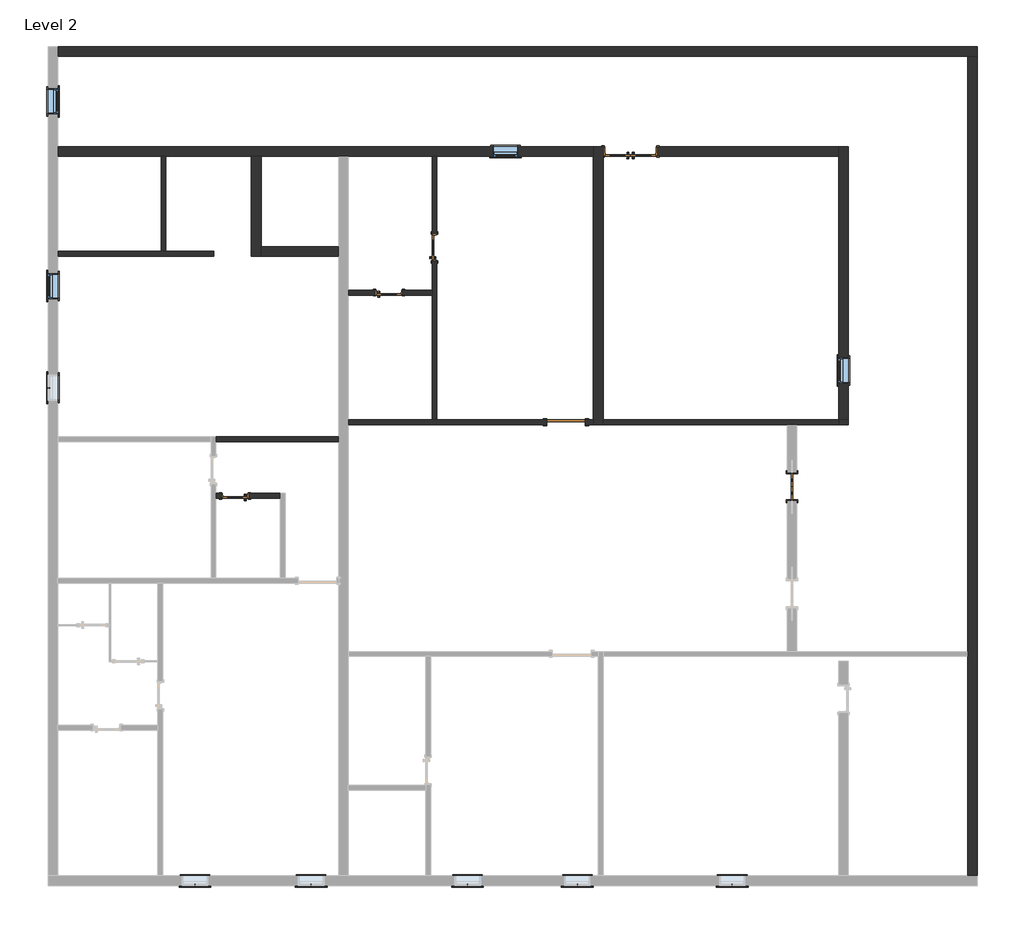
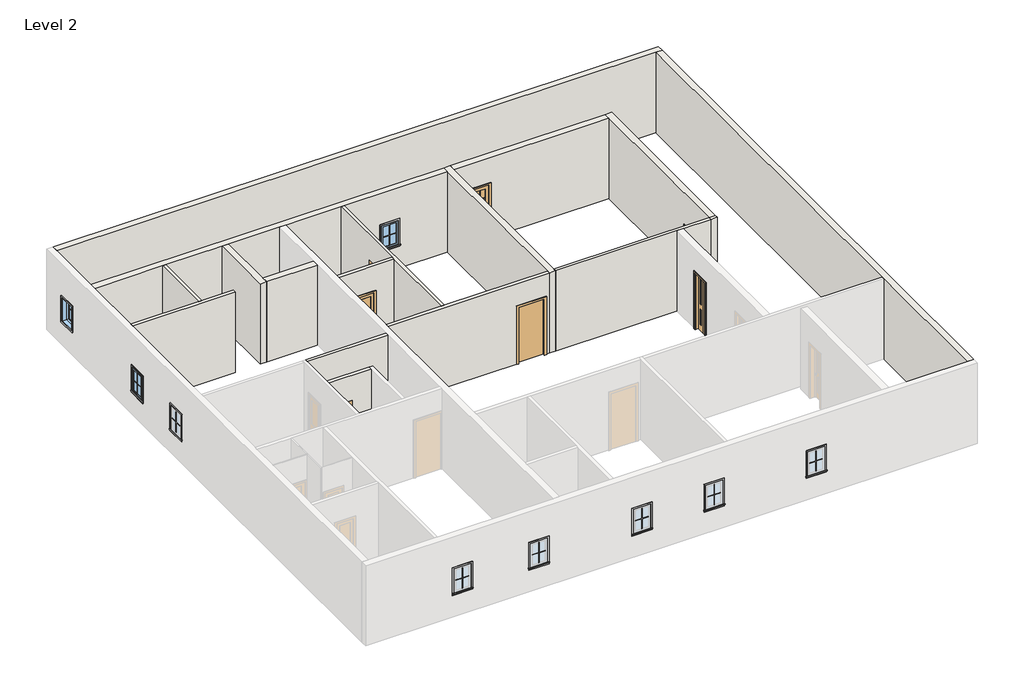
# One storey, part 2 of 2: 30 proxies, 17 walls, 6 doors, 4 windows.
"""IFC4 building model written with IfcOpenShell, lengths in millimetres."""

from ifc_helpers import new_model, si_unit, frame, origin, place, context, project, spatial, polyline, outline, extrude, faceted_brep, transform, mapped, element, save
from components import muntin_pattern_2x2_muntin_pattern_2x2_cf4092f1, muntin_pattern_2x2_muntin_pattern_2x2_49143b38, trim_window_exterior_flat_with_sill_a665a915, trim_window_exterior_flat_with_sill_4c72db77, trim_window_interior_flat_picture_frame_d485c387, trim_window_interior_flat_picture_frame_dfd23ff3, door_cd3c5da8, door_interior_double_pocket_2_panel_wood_door_interior_52fbc1e8, door_interior_single_2_panel_wood_door_interior_single_2_a051e6ed, door_interior_single_2_panel_wood_door_interior_single_2_03d66c98, door_e5f9f3c4, window_bab9308a

model = new_model("IFC4")

# Units and contexts
model_context = context("Model", 3, world=origin())
ifc_project = project(units=[si_unit("LENGTHUNIT", "METRE", prefix="MILLI")], contexts=[model_context])

# Site, building, storey
site = spatial("IfcSite", under=ifc_project)
building = spatial("IfcBuilding", under=site)
storey = spatial("IfcBuildingStorey", under=building, Name="Level 2", Elevation=457.2)

# Proxies
placement = place(None, origin())
muntin_pattern_2x2_muntin_pattern_2x2_shape = muntin_pattern_2x2_muntin_pattern_2x2_cf4092f1(model_context)
element("IfcBuildingElementProxy", 1, Name="Muntin Pattern_2x2 : Muntin Pattern_2x2", ObjectType="Muntin Pattern_2x2 : Muntin Pattern_2x2", at=placement, inside=storey, context=model_context, shape_type="MappedRepresentation", body=[
    mapped(muntin_pattern_2x2_muntin_pattern_2x2_shape, transform((536.9549703, -9076.4534081, 1441.45), x_axis=(-1.0, 0.0, 0.0), y_axis=(0.0, -1.0, 0.0), z_axis=(0.0, 0.0, 1.0))),
])
element("IfcBuildingElementProxy", 2, Name="Muntin Pattern_2x2 : Muntin Pattern_2x2", ObjectType="Muntin Pattern_2x2 : Muntin Pattern_2x2", at=placement, inside=storey, context=model_context, shape_type="MappedRepresentation", body=[
    mapped(muntin_pattern_2x2_muntin_pattern_2x2_shape, transform((-2053.8450297, -9076.4534081, 1441.45), x_axis=(-1.0, 0.0, 0.0), y_axis=(0.0, -1.0, 0.0), z_axis=(0.0, 0.0, 1.0))),
])
element("IfcBuildingElementProxy", 3, Name="Muntin Pattern_2x2 : Muntin Pattern_2x2", ObjectType="Muntin Pattern_2x2 : Muntin Pattern_2x2", at=placement, inside=storey, context=model_context, shape_type="MappedRepresentation", body=[
    mapped(muntin_pattern_2x2_muntin_pattern_2x2_shape, transform((-5749.5450297, -9076.4534081, 1441.45), x_axis=(-1.0, 0.0, 0.0), y_axis=(0.0, -1.0, 0.0), z_axis=(0.0, 0.0, 1.0))),
])
element("IfcBuildingElementProxy", 4, Name="Muntin Pattern_2x2 : Muntin Pattern_2x2", ObjectType="Muntin Pattern_2x2 : Muntin Pattern_2x2", at=placement, inside=storey, context=model_context, shape_type="MappedRepresentation", body=[
    mapped(muntin_pattern_2x2_muntin_pattern_2x2_shape, transform((-8492.7450297, -9076.4534081, 1441.45), x_axis=(-1.0, 0.0, 0.0), y_axis=(0.0, -1.0, 0.0), z_axis=(0.0, 0.0, 1.0))),
])
element("IfcBuildingElementProxy", 5, Name="Muntin Pattern_2x2 : Muntin Pattern_2x2", ObjectType="Muntin Pattern_2x2 : Muntin Pattern_2x2", at=placement, inside=storey, context=model_context, shape_type="MappedRepresentation", body=[
    mapped(muntin_pattern_2x2_muntin_pattern_2x2_shape, transform((-11740.7700297, 9432.2090919, 1441.45), x_axis=(0.0, -1.0, 0.0), y_axis=(1.0, 0.0, 0.0), z_axis=(0.0, 0.0, 1.0))),
])
element("IfcBuildingElementProxy", 6, Name="Muntin Pattern_2x2 : Muntin Pattern_2x2", ObjectType="Muntin Pattern_2x2 : Muntin Pattern_2x2", at=placement, inside=storey, context=model_context, shape_type="MappedRepresentation", body=[
    mapped(muntin_pattern_2x2_muntin_pattern_2x2_shape, transform((-11950.3200297, 5069.7590919, 1441.45), x_axis=(0.0, 1.0, 0.0), y_axis=(-1.0, 0.0, 0.0), z_axis=(0.0, 0.0, 1.0))),
])
element("IfcBuildingElementProxy", 7, Name="Muntin Pattern_2x2 : Muntin Pattern_2x2", ObjectType="Muntin Pattern_2x2 : Muntin Pattern_2x2", at=placement, inside=storey, context=model_context, shape_type="MappedRepresentation", body=[
    mapped(muntin_pattern_2x2_muntin_pattern_2x2_shape, transform((-11950.3200297, 2669.4590919, 1441.45), x_axis=(0.0, 1.0, 0.0), y_axis=(-1.0, 0.0, 0.0), z_axis=(0.0, 0.0, 1.0))),
])
element("IfcBuildingElementProxy", 8, Name="Muntin Pattern_2x2 : Muntin Pattern_2x2", ObjectType="Muntin Pattern_2x2 : Muntin Pattern_2x2", at=placement, inside=storey, context=model_context, shape_type="MappedRepresentation", body=[
    mapped(muntin_pattern_2x2_muntin_pattern_2x2_shape, transform((-1158.4950297, 8146.3340919, 1441.45), x_axis=(-1.0, 0.0, 0.0), y_axis=(0.0, -1.0, 0.0), z_axis=(0.0, 0.0, 1.0))),
])
element("IfcBuildingElementProxy", 9, Name="Muntin Pattern_2x2 : Muntin Pattern_2x2", ObjectType="Muntin Pattern_2x2 : Muntin Pattern_2x2", at=placement, inside=storey, context=model_context, shape_type="MappedRepresentation", body=[
    mapped(muntin_pattern_2x2_muntin_pattern_2x2_shape, transform((6718.6799703, 3075.8590919, 1441.45), x_axis=(0.0, 1.0, 0.0), y_axis=(-1.0, 0.0, 0.0), z_axis=(0.0, 0.0, 1.0))),
])
muntin_pattern_2x2_muntin_pattern_2x2_2_shape = muntin_pattern_2x2_muntin_pattern_2x2_49143b38(model_context)
element("IfcBuildingElementProxy", 10, Name="Muntin Pattern_2x2 : Muntin Pattern_2x2", ObjectType="Muntin Pattern_2x2 : Muntin Pattern_2x2", at=placement, inside=storey, context=model_context, shape_type="MappedRepresentation", body=[
    mapped(muntin_pattern_2x2_muntin_pattern_2x2_2_shape, transform((4194.5549703, -9076.4534081, 1441.45), x_axis=(1.0, 0.0, 0.0), y_axis=(0.0, 1.0, 0.0), z_axis=(0.0, 0.0, 1.0))),
])
trim_window_exterior_flat_with_sill_shape = trim_window_exterior_flat_with_sill_a665a915(model_context)
element("IfcBuildingElementProxy", 11, Name="Trim-Window-Exterior-Flat : with Sill", ObjectType="Trim-Window-Exterior-Flat : with Sill", at=placement, inside=storey, context=model_context, shape_type="MappedRepresentation", body=[
    mapped(trim_window_exterior_flat_with_sill_shape, transform((536.9549703, -9085.9784081, 2286.0), x_axis=(1.0, 0.0, 0.0), y_axis=(0.0, 0.0, 1.0), z_axis=(0.0, -1.0, 0.0))),
])
element("IfcBuildingElementProxy", 12, Name="Trim-Window-Exterior-Flat : with Sill", ObjectType="Trim-Window-Exterior-Flat : with Sill", at=placement, inside=storey, context=model_context, shape_type="MappedRepresentation", body=[
    mapped(trim_window_exterior_flat_with_sill_shape, transform((-2053.8450297, -9085.9784081, 2286.0), x_axis=(1.0, 0.0, 0.0), y_axis=(0.0, 0.0, 1.0), z_axis=(0.0, -1.0, 0.0))),
])
element("IfcBuildingElementProxy", 13, Name="Trim-Window-Exterior-Flat : with Sill", ObjectType="Trim-Window-Exterior-Flat : with Sill", at=placement, inside=storey, context=model_context, shape_type="MappedRepresentation", body=[
    mapped(trim_window_exterior_flat_with_sill_shape, transform((-5749.5450297, -9085.9784081, 2286.0), x_axis=(1.0, 0.0, 0.0), y_axis=(0.0, 0.0, 1.0), z_axis=(0.0, -1.0, 0.0))),
])
element("IfcBuildingElementProxy", 14, Name="Trim-Window-Exterior-Flat : with Sill", ObjectType="Trim-Window-Exterior-Flat : with Sill", at=placement, inside=storey, context=model_context, shape_type="MappedRepresentation", body=[
    mapped(trim_window_exterior_flat_with_sill_shape, transform((-8492.7450297, -9085.9784081, 2286.0), x_axis=(1.0, 0.0, 0.0), y_axis=(0.0, 0.0, 1.0), z_axis=(0.0, -1.0, 0.0))),
])
element("IfcBuildingElementProxy", 15, Name="Trim-Window-Exterior-Flat : with Sill", ObjectType="Trim-Window-Exterior-Flat : with Sill", at=placement, inside=storey, context=model_context, shape_type="MappedRepresentation", body=[
    mapped(trim_window_exterior_flat_with_sill_shape, transform((-11731.2450297, 9432.2090919, 2286.0), x_axis=(0.0, 1.0, 0.0), y_axis=(0.0, 0.0, 1.0), z_axis=(1.0, 0.0, 0.0))),
])
element("IfcBuildingElementProxy", 16, Name="Trim-Window-Exterior-Flat : with Sill", ObjectType="Trim-Window-Exterior-Flat : with Sill", at=placement, inside=storey, context=model_context, shape_type="MappedRepresentation", body=[
    mapped(trim_window_exterior_flat_with_sill_shape, transform((-11959.8450297, 5069.7590919, 2286.0), x_axis=(0.0, -1.0, 0.0), y_axis=(0.0, 0.0, 1.0), z_axis=(-1.0, 0.0, 0.0))),
])
element("IfcBuildingElementProxy", 17, Name="Trim-Window-Exterior-Flat : with Sill", ObjectType="Trim-Window-Exterior-Flat : with Sill", at=placement, inside=storey, context=model_context, shape_type="MappedRepresentation", body=[
    mapped(trim_window_exterior_flat_with_sill_shape, transform((-11959.8450297, 2669.4590919, 2286.0), x_axis=(0.0, -1.0, 0.0), y_axis=(0.0, 0.0, 1.0), z_axis=(-1.0, 0.0, 0.0))),
])
element("IfcBuildingElementProxy", 18, Name="Trim-Window-Exterior-Flat : with Sill", ObjectType="Trim-Window-Exterior-Flat : with Sill", at=placement, inside=storey, context=model_context, shape_type="MappedRepresentation", body=[
    mapped(trim_window_exterior_flat_with_sill_shape, transform((-1158.4950297, 8136.8090919, 2286.0), x_axis=(1.0, 0.0, 0.0), y_axis=(0.0, 0.0, 1.0), z_axis=(0.0, -1.0, 0.0))),
])
element("IfcBuildingElementProxy", 19, Name="Trim-Window-Exterior-Flat : with Sill", ObjectType="Trim-Window-Exterior-Flat : with Sill", at=placement, inside=storey, context=model_context, shape_type="MappedRepresentation", body=[
    mapped(trim_window_exterior_flat_with_sill_shape, transform((6709.1549703, 3075.8590919, 2286.0), x_axis=(0.0, -1.0, 0.0), y_axis=(0.0, 0.0, 1.0), z_axis=(-1.0, 0.0, 0.0))),
])
trim_window_exterior_flat_with_sill_2_shape = trim_window_exterior_flat_with_sill_4c72db77(model_context)
element("IfcBuildingElementProxy", 20, Name="Trim-Window-Exterior-Flat : with Sill", ObjectType="Trim-Window-Exterior-Flat : with Sill", at=placement, inside=storey, context=model_context, shape_type="MappedRepresentation", body=[
    mapped(trim_window_exterior_flat_with_sill_2_shape, transform((4194.5549703, -9085.9784081, 2286.0), x_axis=(-1.0, 0.0, 0.0), y_axis=(0.0, 0.0, -1.0), z_axis=(0.0, -1.0, 0.0))),
])
trim_window_interior_flat_picture_frame_shape = trim_window_interior_flat_picture_frame_d485c387(model_context)
element("IfcBuildingElementProxy", 21, Name="Trim-Window-Interior-Flat : Picture Frame", ObjectType="Trim-Window-Interior-Flat : Picture Frame", at=placement, inside=storey, context=model_context, shape_type="MappedRepresentation", body=[
    mapped(trim_window_interior_flat_picture_frame_shape, transform((536.9549703, -8857.3784081, 2286.0), x_axis=(-1.0, 0.0, 0.0), y_axis=(0.0, 0.0, 1.0), z_axis=(0.0, 1.0, 0.0))),
])
element("IfcBuildingElementProxy", 22, Name="Trim-Window-Interior-Flat : Picture Frame", ObjectType="Trim-Window-Interior-Flat : Picture Frame", at=placement, inside=storey, context=model_context, shape_type="MappedRepresentation", body=[
    mapped(trim_window_interior_flat_picture_frame_shape, transform((-2053.8450297, -8857.3784081, 2286.0), x_axis=(-1.0, 0.0, 0.0), y_axis=(0.0, 0.0, 1.0), z_axis=(0.0, 1.0, 0.0))),
])
element("IfcBuildingElementProxy", 23, Name="Trim-Window-Interior-Flat : Picture Frame", ObjectType="Trim-Window-Interior-Flat : Picture Frame", at=placement, inside=storey, context=model_context, shape_type="MappedRepresentation", body=[
    mapped(trim_window_interior_flat_picture_frame_shape, transform((-5749.5450297, -8857.3784081, 2286.0), x_axis=(-1.0, 0.0, 0.0), y_axis=(0.0, 0.0, 1.0), z_axis=(0.0, 1.0, 0.0))),
])
element("IfcBuildingElementProxy", 24, Name="Trim-Window-Interior-Flat : Picture Frame", ObjectType="Trim-Window-Interior-Flat : Picture Frame", at=placement, inside=storey, context=model_context, shape_type="MappedRepresentation", body=[
    mapped(trim_window_interior_flat_picture_frame_shape, transform((-8492.7450297, -8857.3784081, 2286.0), x_axis=(-1.0, 0.0, 0.0), y_axis=(0.0, 0.0, 1.0), z_axis=(0.0, 1.0, 0.0))),
])
element("IfcBuildingElementProxy", 25, Name="Trim-Window-Interior-Flat : Picture Frame", ObjectType="Trim-Window-Interior-Flat : Picture Frame", at=placement, inside=storey, context=model_context, shape_type="MappedRepresentation", body=[
    mapped(trim_window_interior_flat_picture_frame_shape, transform((-11959.8450297, 9432.2090919, 2286.0), x_axis=(0.0, -1.0, 0.0), y_axis=(0.0, 0.0, 1.0), z_axis=(-1.0, 0.0, 0.0))),
])
element("IfcBuildingElementProxy", 26, Name="Trim-Window-Interior-Flat : Picture Frame", ObjectType="Trim-Window-Interior-Flat : Picture Frame", at=placement, inside=storey, context=model_context, shape_type="MappedRepresentation", body=[
    mapped(trim_window_interior_flat_picture_frame_shape, transform((-11731.2450297, 5069.7590919, 2286.0), x_axis=(0.0, 1.0, 0.0), y_axis=(0.0, 0.0, 1.0), z_axis=(1.0, 0.0, 0.0))),
])
element("IfcBuildingElementProxy", 27, Name="Trim-Window-Interior-Flat : Picture Frame", ObjectType="Trim-Window-Interior-Flat : Picture Frame", at=placement, inside=storey, context=model_context, shape_type="MappedRepresentation", body=[
    mapped(trim_window_interior_flat_picture_frame_shape, transform((-11731.2450297, 2669.4590919, 2286.0), x_axis=(0.0, 1.0, 0.0), y_axis=(0.0, 0.0, 1.0), z_axis=(1.0, 0.0, 0.0))),
])
element("IfcBuildingElementProxy", 28, Name="Trim-Window-Interior-Flat : Picture Frame", ObjectType="Trim-Window-Interior-Flat : Picture Frame", at=placement, inside=storey, context=model_context, shape_type="MappedRepresentation", body=[
    mapped(trim_window_interior_flat_picture_frame_shape, transform((-1158.4950297, 8365.4090919, 2286.0), x_axis=(-1.0, 0.0, 0.0), y_axis=(0.0, 0.0, 1.0), z_axis=(0.0, 1.0, 0.0))),
])
element("IfcBuildingElementProxy", 29, Name="Trim-Window-Interior-Flat : Picture Frame", ObjectType="Trim-Window-Interior-Flat : Picture Frame", at=placement, inside=storey, context=model_context, shape_type="MappedRepresentation", body=[
    mapped(trim_window_interior_flat_picture_frame_shape, transform((6937.7549703, 3075.8590919, 2286.0), x_axis=(0.0, 1.0, 0.0), y_axis=(0.0, 0.0, 1.0), z_axis=(1.0, 0.0, 0.0))),
])
trim_window_interior_flat_picture_frame_2_shape = trim_window_interior_flat_picture_frame_dfd23ff3(model_context)
element("IfcBuildingElementProxy", 30, Name="Trim-Window-Interior-Flat : Picture Frame", ObjectType="Trim-Window-Interior-Flat : Picture Frame", at=placement, inside=storey, context=model_context, shape_type="MappedRepresentation", body=[
    mapped(trim_window_interior_flat_picture_frame_2_shape, transform((4194.5549703, -8857.3784081, 2286.0), x_axis=(1.0, 0.0, 0.0), y_axis=(0.0, 0.0, -1.0), z_axis=(0.0, 1.0, 0.0))),
])

# Doors
door_shape = door_cd3c5da8(model_context)
element("IfcDoor", 31, ObjectType="Door-Interior-Double-Full Glass-Wood : 48\" x 80\"", at=placement, inside=storey, context=model_context, shape_type="MappedRepresentation", body=[
    mapped(door_shape, transform((1794.2549703, 8247.9340919, 457.2), x_axis=(-1.0, 0.0, 0.0), y_axis=(0.0, -1.0, 0.0), z_axis=(0.0, 0.0, 1.0))),
])
door_interior_double_pocket_2_panel_wood_door_interior_shape = door_interior_double_pocket_2_panel_wood_door_interior_52fbc1e8(model_context)
element("IfcDoor", 32, ObjectType="Door-Interior-Double-Pocket-2_Panel-Wood : Door-Interior-Double-Pocket-2_Panel-Wood", at=placement, inside=storey, context=model_context, shape_type="MappedRepresentation", body=[
    mapped(door_interior_double_pocket_2_panel_wood_door_interior_shape, transform((5604.2549703, 332.6590919, 457.2), x_axis=(0.0, -1.0, 0.0), y_axis=(1.0, 0.0, 0.0), z_axis=(0.0, 0.0, 1.0))),
])
door_interior_single_2_panel_wood_door_interior_single_2_shape = door_interior_single_2_panel_wood_door_interior_single_2_a051e6ed(model_context)
element("IfcDoor", 33, ObjectType="Door-Interior-Single-2_Panel-Wood : Door-Interior-Single-2_Panel-Wood", at=placement, inside=storey, context=model_context, shape_type="MappedRepresentation", body=[
    mapped(door_interior_single_2_panel_wood_door_interior_single_2_shape, transform((-7546.5950297, 113.5840919, 457.2), x_axis=(-1.0, 0.0, 0.0), y_axis=(0.0, -1.0, 0.0), z_axis=(0.0, 0.0, 1.0))),
])
element("IfcDoor", 34, ObjectType="Door-Interior-Single-2_Panel-Wood : d3", at=placement, inside=storey, context=model_context, shape_type="MappedRepresentation", body=[
    mapped(door_interior_single_2_panel_wood_door_interior_single_2_shape, transform((-2838.0700297, 5984.1590919, 457.2), x_axis=(0.0, 1.0, 0.0), y_axis=(-1.0, 0.0, 0.0), z_axis=(0.0, 0.0, 1.0))),
])
door_interior_single_2_panel_wood_door_interior_single_2_2_shape = door_interior_single_2_panel_wood_door_interior_single_2_03d66c98(model_context)
element("IfcDoor", 35, ObjectType="Door-Interior-Single-2_Panel-Wood : d3", at=placement, inside=storey, context=model_context, shape_type="MappedRepresentation", body=[
    mapped(door_interior_single_2_panel_wood_door_interior_single_2_2_shape, transform((-3911.2200297, 4914.1840919, 457.2), x_axis=(1.0, 0.0, 0.0), y_axis=(0.0, 1.0, 0.0), z_axis=(0.0, 0.0, 1.0))),
])
door_2_shape = door_e5f9f3c4(model_context)
element("IfcDoor", 36, ObjectType="Single-Flush : 36\" x 84\"", at=placement, inside=storey, context=model_context, shape_type="MappedRepresentation", body=[
    mapped(door_2_shape, transform((270.2549703, 1856.6590919, 457.2), x_axis=(1.0, 0.0, 0.0), y_axis=(0.0, 1.0, 0.0), z_axis=(0.0, 0.0, 1.0))),
])

# Walls
element("IfcWall", 37, ObjectType="4.5\" wall", at=placement, inside=storey, context=model_context, shape_type="SweptSolid", body=[
    extrude(outline(polyline([(3505.2, -6473.4450297), (3505.2, -7997.4450297), (457.2, -7997.4450297), (457.2, -7876.7950297), (2514.6, -7876.7950297), (2514.6, -7216.3950297), (457.2, -7216.3950297), (457.2, -6473.4450297), (3505.2, -6473.4450297)])), frame((0.0, 59.6090919, 0.0), z_axis=(0.0, 1.0, 0.0), x_axis=(0.0, 0.0, 1.0)), (0.0, 0.0, 1.0), 114.3),
])
element("IfcWall", 38, ObjectType="4.5\" wall", at=placement, inside=storey, context=model_context, shape_type="SweptSolid", body=[
    extrude(outline(polyline([(-7997.4450297, 1507.4090919), (-5101.8450297, 1507.4090919), (-5101.8450297, 1393.1090919), (-7997.4450297, 1393.1090919), (-7997.4450297, 1507.4090919)])), frame((0.0, 0.0, 457.2), z_axis=(0.0, 0.0, 1.0), x_axis=(1.0, 0.0, 0.0)), (0.0, 0.0, 1.0), 3048.0),
])
element("IfcWall", 39, ObjectType="4.5\" wall", at=placement, inside=storey, context=model_context, shape_type="Brep", body=[
    faceted_brep([(-2892.0450297, 1913.8090919, 3505.2), (-2892.0450297, 4860.2090919, 3505.2), (-2892.0450297, 4974.5090919, 3505.2), (-2892.0450297, 8136.8090919, 3505.2), (-2892.0450297, 8136.8090919, 457.2), (-2892.0450297, 6314.3590919, 457.2), (-2892.0450297, 6314.3590919, 2514.6), (-2892.0450297, 5653.9590919, 2514.6), (-2892.0450297, 5653.9590919, 457.2), (-2892.0450297, 4974.5090919, 457.2), (-2892.0450297, 4860.2090919, 457.2), (-2892.0450297, 1913.8090919, 457.2), (-2777.7450297, 8136.8090919, 3505.2), (-2777.7450297, 1913.8090919, 3505.2), (-2777.7450297, 1913.8090919, 457.2), (-2777.7450297, 5653.9590919, 457.2), (-2777.7450297, 5653.9590919, 2514.6), (-2777.7450297, 6314.3590919, 2514.6), (-2777.7450297, 6314.3590919, 457.2), (-2777.7450297, 8136.8090919, 457.2)], [[[0, 1, 2, 3, 4, 5, 6, 7, 8, 9, 10, 11]], [[12, 13, 14, 15, 16, 17, 18, 19]], [[4, 19, 18, 5]], [[14, 11, 10, 9, 8, 15]], [[3, 2, 1, 0, 13, 12]], [[4, 3, 12, 19]], [[0, 11, 14, 13]], [[17, 6, 5, 18]], [[6, 17, 16, 7]], [[7, 16, 15, 8]]]),
])
element("IfcWall", 40, ObjectType="4.5\" wall", at=placement, inside=storey, context=model_context, shape_type="Brep", body=[
    faceted_brep([(727.4549703, 1799.5090919, 2590.8), (727.4549703, 1799.5090919, 457.2), (917.9549703, 1799.5090919, 457.2), (917.9549703, 1799.5090919, 3505.2), (-4873.2450297, 1799.5090919, 3505.2), (-4873.2450297, 1799.5090919, 457.2), (-186.9450297, 1799.5090919, 457.2), (-186.9450297, 1799.5090919, 2590.8), (917.9549703, 1913.8090919, 457.2), (727.4549703, 1913.8090919, 457.2), (727.4549703, 1913.8090919, 2590.8), (-186.9450297, 1913.8090919, 2590.8), (-186.9450297, 1913.8090919, 457.2), (-2777.7450297, 1913.8090919, 457.2), (-2892.0450297, 1913.8090919, 457.2), (-4873.2450297, 1913.8090919, 457.2), (-4873.2450297, 1913.8090919, 3505.2), (-2892.0450297, 1913.8090919, 3505.2), (-2777.7450297, 1913.8090919, 3505.2), (917.9549703, 1913.8090919, 3505.2)], [[[0, 1, 2, 3, 4, 5, 6, 7]], [[8, 9, 10, 11, 12, 13, 14, 15, 16, 17, 18, 19]], [[6, 5, 15, 14, 13, 12]], [[2, 1, 9, 8]], [[4, 3, 19, 18, 17, 16]], [[5, 4, 16, 15]], [[3, 2, 8, 19]], [[10, 9, 1, 0]], [[11, 10, 0, 7]], [[12, 11, 7, 6]]]),
])
element("IfcWall", 41, ObjectType="4.5\" wall", at=placement, inside=storey, context=model_context, shape_type="SweptSolid", body=[
    extrude(outline(polyline([(3505.2, -2892.0450297), (3505.2, -4873.2450297), (457.2, -4873.2450297), (457.2, -4241.4200297), (2514.6, -4241.4200297), (2514.6, -3581.0200297), (457.2, -3581.0200297), (457.2, -2892.0450297), (3505.2, -2892.0450297)])), frame((0.0, 4860.2090919, 0.0), z_axis=(0.0, 1.0, 0.0), x_axis=(0.0, 0.0, 1.0)), (0.0, 0.0, 1.0), 114.3),
])
element("IfcWall", 42, ObjectType="4.5\" wall", at=placement, inside=storey, context=model_context, shape_type="SweptSolid", body=[
    extrude(outline(polyline([(6937.7549703, 1799.5090919), (6709.1549703, 1799.5090919), (6709.1549703, 1913.8090919), (6937.7549703, 1913.8090919), (6937.7549703, 1799.5090919)])), frame((0.0, 0.0, 457.2), z_axis=(0.0, 0.0, 1.0), x_axis=(1.0, 0.0, 0.0)), (0.0, 0.0, 1.0), 3048.0),
])
element("IfcWall", 43, ObjectType="4.5\" wall", at=placement, inside=storey, context=model_context, shape_type="Brep", body=[
    faceted_brep([(6709.1549703, 1913.8090919, 457.2), (1146.5549703, 1913.8090919, 457.2), (1146.5549703, 1913.8090919, 3505.2), (6709.1549703, 1913.8090919, 3505.2), (6709.1549703, 1799.5090919, 457.2), (6709.1549703, 1799.5090919, 3505.2), (5718.5549703, 1799.5090919, 3505.2), (5489.9549703, 1799.5090919, 3505.2), (1146.5549703, 1799.5090919, 3505.2), (1146.5549703, 1799.5090919, 457.2), (5489.9549703, 1799.5090919, 457.2), (5718.5549703, 1799.5090919, 457.2)], [[[0, 1, 2, 3]], [[4, 5, 6, 7, 8, 9, 10, 11]], [[1, 0, 4, 11, 10, 9]], [[3, 2, 8, 7, 6, 5]], [[0, 3, 5, 4]], [[2, 1, 9, 8]]]),
])
element("IfcWall", 44, ObjectType="4.5\" wall", at=placement, inside=storey, context=model_context, shape_type="SweptSolid", body=[
    extrude(outline(polyline([(-9178.5450297, 8136.8090919), (-9178.5450297, 5888.9090919), (-9292.8450297, 5888.9090919), (-9292.8450297, 8136.8090919), (-9178.5450297, 8136.8090919)])), frame((0.0, 0.0, 457.2), z_axis=(0.0, 0.0, 1.0), x_axis=(1.0, 0.0, 0.0)), (0.0, 0.0, 1.0), 3048.0),
])
element("IfcWall", 45, ObjectType="4.5\" wall", at=placement, inside=storey, context=model_context, shape_type="Brep", body=[
    faceted_brep([(-11731.2450297, 5774.6090919, 457.2), (-8051.366475, 5774.6090919, 457.2), (-8051.366475, 5774.6090919, 3505.2), (-11731.2450297, 5774.6090919, 3505.2), (-11731.2450297, 5888.9090919, 457.2), (-11731.2450297, 5888.9090919, 3505.2), (-9292.8450297, 5888.9090919, 3505.2), (-9178.5450297, 5888.9090919, 3505.2), (-8051.366475, 5888.9090919, 3505.2), (-8051.366475, 5888.9090919, 457.2), (-9178.5450297, 5888.9090919, 457.2), (-9292.8450297, 5888.9090919, 457.2)], [[[0, 1, 2, 3]], [[4, 5, 6, 7, 8, 9, 10, 11]], [[1, 0, 4, 11, 10, 9]], [[2, 1, 9, 8]], [[3, 2, 8, 7, 6, 5]], [[0, 3, 5, 4]]]),
])
element("IfcWall", 46, ObjectType="9\" wall", at=placement, inside=storey, context=model_context, shape_type="Brep", body=[
    faceted_brep([(1146.5549703, 1799.5090919, 457.2), (1146.5549703, 1913.8090919, 457.2), (1146.5549703, 8136.8090919, 457.2), (1146.5549703, 8365.4090919, 457.2), (1146.5549703, 8365.4090919, 3505.2), (1146.5549703, 8136.8090919, 3505.2), (1146.5549703, 1913.8090919, 3505.2), (1146.5549703, 1799.5090919, 3505.2), (917.9549703, 1799.5090919, 457.2), (917.9549703, 1799.5090919, 3505.2), (917.9549703, 1913.8090919, 3505.2), (917.9549703, 8136.8090919, 3505.2), (917.9549703, 8365.4090919, 3505.2), (917.9549703, 8365.4090919, 457.2), (917.9549703, 8136.8090919, 457.2), (917.9549703, 1913.8090919, 457.2)], [[[0, 1, 2, 3, 4, 5, 6, 7]], [[8, 9, 10, 11, 12, 13, 14, 15]], [[3, 2, 1, 0, 8, 15, 14, 13]], [[7, 6, 5, 4, 12, 11, 10, 9]], [[4, 3, 13, 12]], [[0, 7, 9, 8]]]),
])
element("IfcWall", 47, ObjectType="9\" wall", at=placement, inside=storey, context=model_context, shape_type="Brep", body=[
    faceted_brep([(-11731.2450297, 8136.8090919, 457.2), (-9292.8450297, 8136.8090919, 457.2), (-9178.5450297, 8136.8090919, 457.2), (-7159.2450297, 8136.8090919, 457.2), (-6930.6450297, 8136.8090919, 457.2), (-5101.8450297, 8136.8090919, 457.2), (-4873.2450297, 8136.8090919, 457.2), (-2892.0450297, 8136.8090919, 457.2), (-2777.7450297, 8136.8090919, 457.2), (917.9549703, 8136.8090919, 457.2), (917.9549703, 8136.8090919, 3505.2), (-2777.7450297, 8136.8090919, 3505.2), (-2892.0450297, 8136.8090919, 3505.2), (-4873.2450297, 8136.8090919, 3505.2), (-5101.8450297, 8136.8090919, 3505.2), (-6930.6450297, 8136.8090919, 3505.2), (-7159.2450297, 8136.8090919, 3505.2), (-9178.5450297, 8136.8090919, 3505.2), (-9292.8450297, 8136.8090919, 3505.2), (-11731.2450297, 8136.8090919, 3505.2), (-1463.2950297, 8136.8090919, 2286.0), (-853.6950297, 8136.8090919, 2286.0), (-853.6950297, 8136.8090919, 1371.6), (-1463.2950297, 8136.8090919, 1371.6), (-11731.2450297, 8365.4090919, 457.2), (-11731.2450297, 8365.4090919, 3505.2), (917.9549703, 8365.4090919, 3505.2), (917.9549703, 8365.4090919, 457.2), (-1463.2950297, 8365.4090919, 2286.0), (-1463.2950297, 8365.4090919, 1371.6), (-853.6950297, 8365.4090919, 1371.6), (-853.6950297, 8365.4090919, 2286.0)], [[[0, 1, 2, 3, 4, 5, 6, 7, 8, 9, 10, 11, 12, 13, 14, 15, 16, 17, 18, 19], [20, 21, 22, 23]], [[24, 25, 26, 27], [28, 29, 30, 31]], [[9, 8, 7, 6, 5, 4, 3, 2, 1, 0, 24, 27]], [[19, 18, 17, 16, 15, 14, 13, 12, 11, 10, 26, 25]], [[10, 9, 27, 26]], [[0, 19, 25, 24]], [[29, 28, 20, 23]], [[30, 29, 23, 22]], [[31, 30, 22, 21]], [[28, 31, 21, 20]]]),
])
element("IfcWall", 48, ObjectType="9\" wall", at=placement, inside=storey, context=model_context, shape_type="Brep", body=[
    faceted_brep([(6937.7549703, 1913.8090919, 457.2), (6937.7549703, 8365.4090919, 457.2), (6937.7549703, 8365.4090919, 3505.2), (6937.7549703, 1913.8090919, 3505.2), (6937.7549703, 3380.6590919, 2286.0), (6937.7549703, 3380.6590919, 1371.6), (6937.7549703, 2771.0590919, 1371.6), (6937.7549703, 2771.0590919, 2286.0), (6709.1549703, 1913.8090919, 457.2), (6709.1549703, 1913.8090919, 3505.2), (6709.1549703, 8136.8090919, 3505.2), (6709.1549703, 8365.4090919, 3505.2), (6709.1549703, 8365.4090919, 457.2), (6709.1549703, 8136.8090919, 457.2), (6709.1549703, 3380.6590919, 2286.0), (6709.1549703, 2771.0590919, 2286.0), (6709.1549703, 2771.0590919, 1371.6), (6709.1549703, 3380.6590919, 1371.6)], [[[0, 1, 2, 3], [4, 5, 6, 7]], [[8, 9, 10, 11, 12, 13], [14, 15, 16, 17]], [[1, 0, 8, 13, 12]], [[3, 2, 11, 10, 9]], [[2, 1, 12, 11]], [[0, 3, 9, 8]], [[5, 4, 14, 17]], [[6, 5, 17, 16]], [[7, 6, 16, 15]], [[4, 7, 15, 14]]]),
])
element("IfcWall", 49, ObjectType="9\" wall", at=placement, inside=storey, context=model_context, shape_type="SweptSolid", body=[
    extrude(outline(polyline([(3505.2, 6709.1549703), (3505.2, 1146.5549703), (457.2, 1146.5549703), (457.2, 1159.2549703), (2514.6, 1159.2549703), (2514.6, 2429.2549703), (457.2, 2429.2549703), (457.2, 6709.1549703), (3505.2, 6709.1549703)])), frame((0.0, 8136.8090919, 0.0), z_axis=(0.0, 1.0, 0.0), x_axis=(0.0, 0.0, 1.0)), (0.0, 0.0, 1.0), 228.6),
])
element("IfcWall", 50, ObjectType="9\" wall", at=placement, inside=storey, context=model_context, shape_type="Brep", body=[
    faceted_brep([(-6930.6450297, 5774.6090919, 457.2), (-6930.6450297, 6003.2090919, 457.2), (-6930.6450297, 8136.8090919, 457.2), (-6930.6450297, 8136.8090919, 3505.2), (-6930.6450297, 6003.2090919, 3505.2), (-6930.6450297, 5774.6090919, 3505.2), (-7159.2450297, 5774.6090919, 457.2), (-7159.2450297, 5774.6090919, 3505.2), (-7159.2450297, 8136.8090919, 3505.2), (-7159.2450297, 8136.8090919, 457.2)], [[[0, 1, 2, 3, 4, 5]], [[6, 7, 8, 9]], [[2, 1, 0, 6, 9]], [[5, 4, 3, 8, 7]], [[3, 2, 9, 8]], [[0, 5, 7, 6]]]),
])
element("IfcWall", 51, ObjectType="9\" wall", at=placement, inside=storey, context=model_context, shape_type="SweptSolid", body=[
    extrude(outline(polyline([(-5101.8450297, 5774.6090919), (-6930.6450297, 5774.6090919), (-6930.6450297, 6003.2090919), (-5101.8450297, 6003.2090919), (-5101.8450297, 5774.6090919)])), frame((0.0, 0.0, 457.2), z_axis=(0.0, 0.0, 1.0), x_axis=(1.0, 0.0, 0.0)), (0.0, 0.0, 1.0), 3048.0),
])
element("IfcWall", 52, ObjectType="9\" wall", at=placement, inside=storey, context=model_context, shape_type="Brep", body=[
    faceted_brep([(-11731.2450297, 10499.0090919, 457.2), (9757.1549703, 10499.0090919, 457.2), (9985.7549703, 10499.0090919, 457.2), (9985.7549703, 10499.0090919, 3505.2), (9757.1549703, 10499.0090919, 3505.2), (-11731.2450297, 10499.0090919, 3505.2), (-11731.2450297, 10727.6090919, 457.2), (-11731.2450297, 10727.6090919, 3505.2), (9985.7549703, 10727.6090919, 3505.2), (9985.7549703, 10727.6090919, 457.2)], [[[0, 1, 2, 3, 4, 5]], [[6, 7, 8, 9]], [[2, 1, 0, 6, 9]], [[5, 4, 3, 8, 7]], [[0, 5, 7, 6]], [[3, 2, 9, 8]]]),
])
element("IfcWall", 53, ObjectType="9\" wall", at=placement, inside=storey, context=model_context, shape_type="Brep", body=[
    faceted_brep([(9985.7549703, -8855.7909081, 457.2), (9985.7549703, 10499.0090919, 457.2), (9985.7549703, 10499.0090919, 3505.2), (9985.7549703, -8855.7909081, 3505.2), (9757.1549703, -8855.7909081, 457.2), (9757.1549703, -8855.7909081, 3505.2), (9757.1549703, -3674.1909081, 3505.2), (9757.1549703, -3559.8909081, 3505.2), (9757.1549703, 10499.0090919, 3505.2), (9757.1549703, 10499.0090919, 457.2), (9757.1549703, -3559.8909081, 457.2), (9757.1549703, -3674.1909081, 457.2)], [[[0, 1, 2, 3]], [[4, 5, 6, 7, 8, 9, 10, 11]], [[1, 0, 4, 11, 10, 9]], [[3, 2, 8, 7, 6, 5]], [[0, 3, 5, 4]], [[2, 1, 9, 8]]]),
])

# Windows
window_shape = window_bab9308a(model_context)
element("IfcWindow", 54, ObjectType="Window-Casement-Single_Left : 24\" x 36\"", at=placement, inside=storey, context=model_context, shape_type="MappedRepresentation", body=[
    mapped(window_shape, transform((-11845.5450297, 9432.2090919, 457.2), x_axis=(0.0, -1.0, 0.0), y_axis=(1.0, 0.0, 0.0), z_axis=(0.0, 0.0, 1.0))),
])
element("IfcWindow", 55, ObjectType="Window-Casement-Single_Left : 24\" x 36\"", at=placement, inside=storey, context=model_context, shape_type="MappedRepresentation", body=[
    mapped(window_shape, transform((-11845.5450297, 5069.7590919, 457.2), x_axis=(0.0, 1.0, 0.0), y_axis=(-1.0, 0.0, 0.0), z_axis=(0.0, 0.0, 1.0))),
])
element("IfcWindow", 56, ObjectType="Window-Casement-Single_Left : 24\" x 36\"", at=placement, inside=storey, context=model_context, shape_type="MappedRepresentation", body=[
    mapped(window_shape, transform((-1158.4950297, 8251.1090919, 457.2), x_axis=(-1.0, 0.0, 0.0), y_axis=(0.0, -1.0, 0.0), z_axis=(0.0, 0.0, 1.0))),
])
element("IfcWindow", 57, ObjectType="Window-Casement-Single_Left : 24\" x 36\"", at=placement, inside=storey, context=model_context, shape_type="MappedRepresentation", body=[
    mapped(window_shape, transform((6823.4549703, 3075.8590919, 457.2), x_axis=(0.0, 1.0, 0.0), y_axis=(-1.0, 0.0, 0.0), z_axis=(0.0, 0.0, 1.0))),
])

save(model, "model.ifc")

# Revit data of these elements
# Type "Muntin Pattern_2x2 : Muntin Pattern_2x2"
#   Width [instance default] = 4' - 0"
#   Thickness = 0' - 0 1/2"
#   Height [instance default] = 4' - 0"
#   Distance = 0' - 0 3/4"
#   Interior Material [instance default] = none
#   Exterior Material [instance default] = none
#   Default Elevation = 0
# Type "Trim-Window-Exterior-Flat : with Sill"
#   Trim Width = 0' - 2 1/4"
#   Trim Thickness_Picture Frame = 0' - 1 1/4"
#   Trim Thickness_with Sill = 0' - 0 3/4"
#   Sill Thickness = 0' - 1 1/4"
#   Opening Width [instance default] = 2' - 0"
#   Opening Height [instance default] = 3' - 0"
#   Default Elevation = 4' - 0"
#   Sill = yes
#   Picture Frame = no
#   Trim Material [instance default] = none
# Type "Trim-Window-Interior-Flat : Picture Frame"
#   Trim Thickness_Picture Frame = 0' - 1 1/4"
#   Trim Width = 0' - 2 1/4"
#   Trim Thickness_with Sill = 0' - 0 3/4"
#   Sill Thickness = 0' - 1 1/4"
#   Opening Width [instance default] = 2' - 0"
#   Opening Height [instance default] = 3' - 0"
#   Default Elevation = 4' - 0"
#   Sill = no
#   Picture Frame = yes
#   Trim Material [instance default] = none
# Type "Door-Interior-Double-Full Glass-Wood : 48\" x 80\""
#   Type Mark = "11"
#   Assembly Code = "C1020300"
#   Analytic Construction = "French door, wood frame with single glass"
#   Top Rail = 0' - 4 11/16"
#   Thickness = 0' - 1 3/8"
#   Thermal Resistance (R) = 1.0696 (h·ft²·°F)/BTU
#   Swing Angle [instance default] = 90.00°
#   Stiles = 0' - 4 3/4"
#   Rough Width = 4' - 2"
#   Rough Height = 6' - 9"
#   Panel Width = 2' - 0"
#   Height = 6' - 8"
#   Width = 4' - 0"
#   Heat Transfer Coefficient (U) = 0.9350 BTU/(h·ft²·°F)
#   Bottom Rail = 0' - 9 1/8"
#   Show Grill [instance default] = yes
#   Trim Material = Cherry
#   Panel Material = Cherry
#   Frame Material = Cherry
#   Door Handle Material = Aluminum
#   Visual Light Transmittance = 0
#   Solar Heat Gain Coefficient = 0
#   Wall Closure = (empty or 0)
#   Function = (empty or 0)
# Type "Door-Interior-Double-Pocket-2_Panel-Wood : Door-Interior-Double-Pocket-2_Panel-Wood"
#   Type Mark = "14"
#   Assembly Code = "C1020300"
#   Analytic Construction = "Wooden"
#   Top Rail = 0' - 4 11/16"
#   Thickness = 0' - 1 3/8"
#   Thermal Resistance (R) = 2.5876 (h·ft²·°F)/BTU
#   Stiles = 0' - 4 3/4"
#   Rough Width = 4' - 2"
#   Rough Height = 7' - 4 1/2"
#   Panel Width = 1' - 0"
#   Lock Rail = 0' - 7 1/2"
#   Location [instance default] = 1' - 1"
#   Height = 7' - 0"
#   Width = 2' - 0"
#   Heat Transfer Coefficient (U) = 0.3865 BTU/(h·ft²·°F)
#   Bottom Rail = 0' - 9 1/8"
#   Panel Open [instance default] = no
#   Trim Material = Cherry
#   Panel Material = Cherry
#   Frame Material = Cherry
#   Visual Light Transmittance = 0
#   Solar Heat Gain Coefficient = 0
#   Wall Closure = (empty or 0)
#   Function = (empty or 0)
# Type "Door-Interior-Single-2_Panel-Wood : Door-Interior-Single-2_Panel-Wood"
#   Type Mark = "12"
#   Assembly Code = "C1020300"
#   Analytic Construction = "Wooden"
#   Top Rail = 0' - 4 11/16"
#   Thickness = 0' - 1 3/8"
#   Thermal Resistance (R) = 2.5876 (h·ft²·°F)/BTU
#   Swing Angle [instance default] = 90.00°
#   Stiles = 0' - 4 3/4"
#   Rough Width = 2' - 2"
#   Rough Height = 6' - 9"
#   Lock Rail = 0' - 7 1/2"
#   Height = 6' - 8"
#   Width = 2' - 0"
#   Heat Transfer Coefficient (U) = 0.3865 BTU/(h·ft²·°F)
#   Bottom Rail = 0' - 9 1/8"
#   Trim Material = Cherry
#   Panel Material = Cherry
#   Frame Material = Cherry
#   Door Handle Material = Aluminum
#   Visual Light Transmittance = 0
#   Solar Heat Gain Coefficient = 0
#   Wall Closure = (empty or 0)
#   Function = (empty or 0)
# Type "Door-Interior-Single-2_Panel-Wood : d3"
#   Type Mark = "13"
#   Assembly Code = "C1020300"
#   Analytic Construction = "Wooden"
#   Top Rail = 0' - 4 11/16"
#   Thickness = 0' - 1 3/8"
#   Thermal Resistance (R) = 2.5876 (h·ft²·°F)/BTU
#   Swing Angle [instance default] = 90.00°
#   Stiles = 0' - 4 3/4"
#   Rough Width = 2' - 2"
#   Rough Height = 6' - 9"
#   Lock Rail = 0' - 7 1/2"
#   Height = 6' - 8"
#   Width = 2' - 0"
#   Heat Transfer Coefficient (U) = 0.3865 BTU/(h·ft²·°F)
#   Bottom Rail = 0' - 9 1/8"
#   Trim Material = Cherry
#   Panel Material = Cherry
#   Frame Material = Cherry
#   Door Handle Material = Aluminum
#   Visual Light Transmittance = 0
#   Solar Heat Gain Coefficient = 0
#   Wall Closure = (empty or 0)
#   Function = (empty or 0)
# Type "Single-Flush : 36\" x 84\""
#   Type Mark = "1"
#   Construction Type Id = "MDOOR"
#   Assembly Code = "C1020"
#   Analytic Construction = "Metal"
#   Thickness = 0' - 2"
#   Heat Transfer Coefficient (U) = 0.651978 BTU/(h·ft²·°F)
#   Height = 7' - 0"
#   Trim Projection Ext = 0' - 1"
#   Trim Projection Int = 0' - 1"
#   Trim Width = 0' - 3"
#   Width = 3' - 0"
#   Define Thermal Properties by = 1
#   Define Thermal Properties by = 1
#   Door Material = Door - Panel
#   Frame Material = Door - Frame
#   Visual Light Transmittance = 0
#   Solar Heat Gain Coefficient = 0
#   Function = (empty or 0)
#   Wall Closure = (empty or 0)
# Type "4.5\" wall"
#   Assembly Code = "B2010"
#   Layers, outside or top first: 0' - 4 1/2" no material (function 1)
# Type "9\" wall"
#   Assembly Code = "B2010"
#   Layers, outside or top first: 0' - 9" no material (function 1)
# Type "Window-Casement-Single_Left : 24\" x 36\""
#   Type Mark = "18"
#   Fire Rating = "0.5h"
#   Assembly Code = "B2020100"
#   Analytic Construction = "Double glazing - domestic"
#   Window Inset [instance default] = 0' - 0"
#   Wall Thickness [instance default] = 0' - 6"
#   Visual Light Transmittance = 0.81
#   Thermal Resistance (R) = 1.8146 (h·ft²·°F)/BTU
#   Solar Heat Gain Coefficient = 0.76
#   Rough Width = 2' - 0 1/2"
#   Rough Height = 3' - 0 1/2"
#   Interior Wall Closure [instance default] = 0' - 2 1/4"
#   Height = 3' - 0"
#   Heat Transfer Coefficient (U) = 0.5511 BTU/(h·ft²·°F)
#   Frame Extension [instance default] = 0' - 0 1/4"
#   Exterior Wall Closure [instance default] = 0' - 1 1/4"
#   Extension Jamb [instance default] = 0' - 2 1/4"
#   Default Sill Height = 3' - 0"
#   Width = 2' - 0"
#   Muntin Visibility = yes
#   Interior Trim Visibility [instance default] = yes
#   Exterior Trim Visibility [instance default] = yes
#   Extension Jamb Visibility [instance default] = yes
#   Muntin Pattern = Muntin Pattern_2x2 : Muntin Pattern_2x2
#   Interior Trim Material = Wood - Stained
#   Interior Trim = Trim-Window-Interior-Flat : Picture Frame
#   Interior Frame Material = Wood - Stained
#   Glass Panel Material = Glass
#   Exterior Trim Material = Clad - White
#   Exterior Trim = Trim-Window-Exterior-Flat : with Sill
#   Exterior Frame Material = Clad - White
#   Wall Closure = (empty or 0)
# Elements 1, 2, 3, 4, 5, 6, 7, 8, 9, 10 (IfcBuildingElementProxy, "Muntin Pattern_2x2 : Muntin Pattern_2x2")
#   Width = 1' - 6 1/2"
#   Height = 2' - 6 1/2"
#   Interior Material = Wood - Stained
#   Exterior Material = Clad - White
#   Phase Created = New Construction
#   Materials on its faces: "Clad - White", "Wood - Stained"
# Elements 11, 12, 13, 14, 15, 16, 17, 18, 19, 20 (IfcBuildingElementProxy, "Trim-Window-Exterior-Flat : with Sill")
#   Opening Width = 2' - 0"
#   Opening Height = 3' - 0"
#   Trim Material = Clad - White
#   Phase Created = New Construction
#   Materials on its faces: "Clad - White"
# Elements 21, 22, 23, 24, 25, 26, 27, 28, 29, 30 (IfcBuildingElementProxy, "Trim-Window-Interior-Flat : Picture Frame")
#   Opening Width = 2' - 0"
#   Opening Height = 3' - 0"
#   Trim Material = Wood - Stained
#   Phase Created = New Construction
#   Materials on its faces: "Wood - Stained"
# Element 31 (IfcDoor, "Door-Interior-Double-Full Glass-Wood : 48\" x 80\"")
#   Swing Angle = 90.00°
#   Show Grill = yes
#   Phase Created = New Construction
#   Materials on its faces: "Cherry", "Aluminum", "Glass"
# Element 32 (IfcDoor, "Door-Interior-Double-Pocket-2_Panel-Wood : Door-Interior-Double-Pocket-2_Panel-Wood")
#   Location = 1' - 1"
#   Panel Open = no
#   Phase Created = New Construction
#   Materials on its faces: "Cherry"
# Element 33 (IfcDoor, "Door-Interior-Single-2_Panel-Wood : Door-Interior-Single-2_Panel-Wood")
#   Swing Angle = 90.00°
#   Phase Created = New Construction
#   Materials on its faces: "Cherry", "Aluminum"
# Elements 34, 35 (IfcDoor, "Door-Interior-Single-2_Panel-Wood : d3")
#   Swing Angle = 90.00°
#   Phase Created = New Construction
#   Materials on its faces: "Cherry", "Aluminum"
# Element 36 (IfcDoor, "Single-Flush : 36\" x 84\"")
#   Phase Created = New Construction
#   Materials on its faces: "Door - Frame", "Door - Panel"
# Elements 37, 38, 39, 40, 41, 42, 43, 44, 45 (IfcWall, "4.5\" wall")
#   Top Offset = 0' - 0"
#   Base Offset = 0' - 0"
#   wall height = 10' - 0"
#   Phase Created = New Construction
#   Base Constraint = Level 2
#   Top Constraint = Level 3
#   Materials on its faces: "Default Wall"
# Elements 46, 47, 48, 49, 50, 51, 52, 53 (IfcWall, "9\" wall")
#   Top Offset = 0' - 0"
#   Base Offset = 0' - 0"
#   wall height = 10' - 0"
#   Phase Created = New Construction
#   Base Constraint = Level 2
#   Top Constraint = Level 3
#   Materials on its faces: "Default Wall"
# Element 54 (IfcWindow, "Window-Casement-Single_Left : 24\" x 36\"")
#   Mark = "6"
#   Window Inset = 0' - 0"
#   Interior Wall Closure = 0' - 2 1/4"
#   Frame Extension = 0' - 0 1/4"
#   Exterior Wall Closure = 0' - 1 1/4"
#   Interior Trim Visibility = yes
#   Exterior Trim Visibility = yes
#   Phase Created = New Construction
#   Materials on its faces: "Wood - Stained", "Glass", "Clad - White"
# Element 55 (IfcWindow, "Window-Casement-Single_Left : 24\" x 36\"")
#   Mark = "7"
#   Window Inset = 0' - 0"
#   Interior Wall Closure = 0' - 2 1/4"
#   Frame Extension = 0' - 0 1/4"
#   Exterior Wall Closure = 0' - 1 1/4"
#   Interior Trim Visibility = yes
#   Exterior Trim Visibility = yes
#   Phase Created = New Construction
#   Materials on its faces: "Wood - Stained", "Glass", "Clad - White"
# Element 56 (IfcWindow, "Window-Casement-Single_Left : 24\" x 36\"")
#   Mark = "9"
#   Window Inset = 0' - 0"
#   Interior Wall Closure = 0' - 2 1/4"
#   Frame Extension = 0' - 0 1/4"
#   Exterior Wall Closure = 0' - 1 1/4"
#   Interior Trim Visibility = yes
#   Exterior Trim Visibility = yes
#   Phase Created = New Construction
#   Materials on its faces: "Wood - Stained", "Glass", "Clad - White"
# Element 57 (IfcWindow, "Window-Casement-Single_Left : 24\" x 36\"")
#   Mark = "10"
#   Window Inset = 0' - 0"
#   Interior Wall Closure = 0' - 2 1/4"
#   Frame Extension = 0' - 0 1/4"
#   Exterior Wall Closure = 0' - 1 1/4"
#   Interior Trim Visibility = yes
#   Exterior Trim Visibility = yes
#   Phase Created = New Construction
#   Materials on its faces: "Wood - Stained", "Glass", "Clad - White"
# Materials
#   "Cherry": class "Wood", colour RGB 226 177 128, transparency 0, Description = "Prunus Serotina", Cost = 0
#   "Aluminum": class "Metal", colour RGB 247 247 247, transparency 0, Description = "Aluminum 6061", Cost = 0
#   "Door - Panel": class "Wood", colour RGB 210 159 95, transparency 0, Cost = 0
#   "Door - Frame": colour RGB 118 70 51, transparency 0, Cost = 0
#   "Wood - Stained": class "Wood", colour RGB 224 178 126, transparency 0, Cost = 0
#   "Glass": class "Glass", colour RGB 0 128 192, transparency 0.75, Description = "Soda Lime Glass", Cost = 0
#   "Clad - White": class "Wood", colour RGB 242 242 238, transparency 0, Cost = 0
#   "Default Wall": colour RGB 128 128 128, transparency 0, Cost = 0
